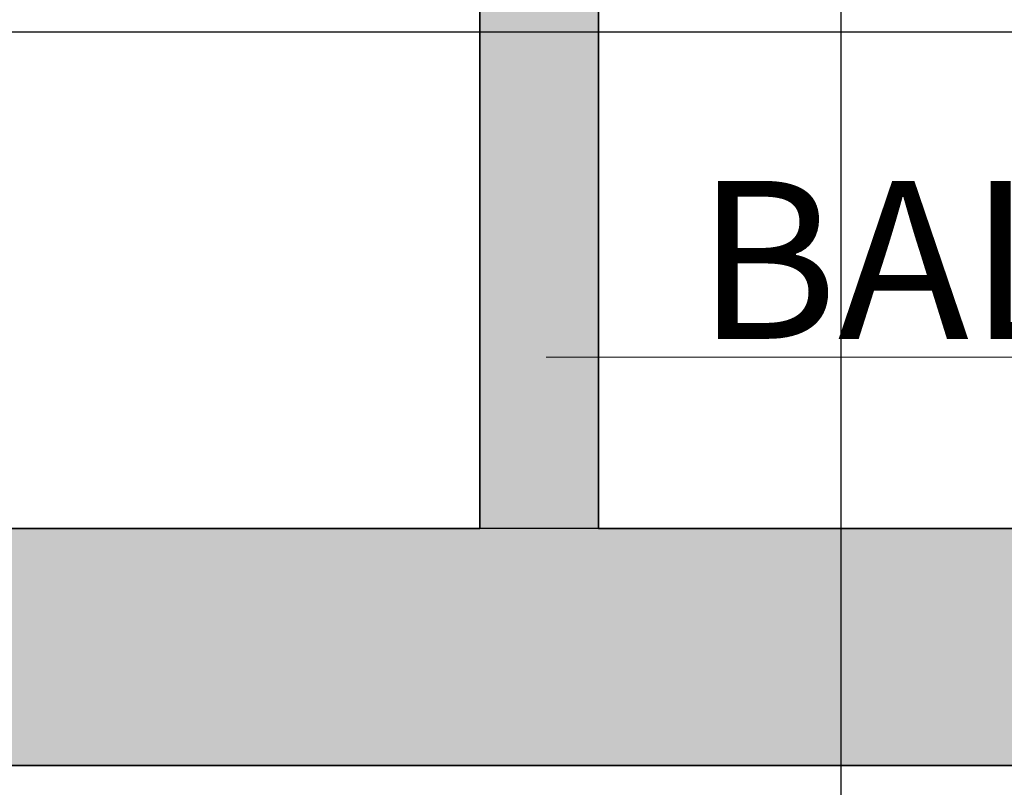
# Model space of a CAD drawing. Units: inches. Extents: x 2696 to 3240, y 1564 to 2310.
# Tile 3 of 76: x 2875 to 2912, y 1604 to 1634. Entities that reach past the tile are written whole.
import ezdxf

# ---------------------------------------------------------------- set-up
doc = ezdxf.new("R2010")
doc.units = ezdxf.units.IN
for name, color, linetype, lineweight in [('A-ANNO-DIMS', 3, 'Continuous', 18), ('A-WALL', 7, 'Continuous', 35), ('A-WALL-PATT', 9, 'Continuous', 13)]:
    doc.layers.add(name, color=color, linetype=linetype, lineweight=lineweight)
doc.styles.add('TIMES NEW', font='times.ttf')
doc.dimstyles.new('Siddhuu', dxfattribs={"dimtxt": 6, "dimasz": 2.5, "dimexe": 1.25, "dimexo": 0.625, "dimtad": 1, "dimdec": 1, "dimlunit": 4, "dimtxsty": 'TIMES NEW', "dimcen": 2.5, "dimclrd": 256, "dimclre": 1, "dimclrt": 7, "dimadec": 0, "dimazin": 0, "dimtfac": 1, "dimtdec": 1, "dimtmove": 0, "dimatfit": 3, "dimfxl": 1, "dimtolj": 1, "dimlwd": -1, "dimarcsym": 0})

# ---------------------------------------------------------------- blocks, each defined once
blk = doc.blocks.new('*D36')
at = {"layer": 'A-ANNO-DIMS', "color": 1, "lineweight": -2, "transparency": 16777216}
for p, q in [((3008.237, 1629.386), (3008.237, 1619.461)), ((3070.237, 1629.386), (3070.237, 1619.461))]:
    blk.add_line(p, q, dxfattribs=at)
at = {"layer": 'A-ANNO-DIMS', "transparency": 16777216}
for p, q in [((3008.237, 1620.711), (2894.718, 1620.711)), ((3067.737, 1620.711), (3010.737, 1620.711))]:
    blk.add_line(p, q, dxfattribs=at)
for points in [[(3010.737, 1621.128), (3010.737, 1620.294), (3008.237, 1620.711)], [(3067.737, 1621.128), (3067.737, 1620.294), (3070.237, 1620.711)]]:
    blk.add_solid(points, dxfattribs=at)
at = {"layer": 'Defpoints', "color": 0, "transparency": 16777216}
for p in [(3008.237, 1630.011), (3070.237, 1630.011), (3008.237, 1620.711)]:
    blk.add_point(p, dxfattribs=at)
at = {"layer": 'A-ANNO-DIMS', "color": 7, "transparency": 16777216, "insert": (2950.228, 1624.403), "char_height": 6, "attachment_point": 5, "style": 'TIMES NEW'}
blk.add_mtext('\\A1;BALCONY DOOR 5\'-2" TYP.', dxfattribs=at)
blk = doc.blocks.new('*D57')
at = {"layer": 'A-ANNO-DIMS', "color": 1, "lineweight": -2, "transparency": 16777216}
for p, q in [((2754.611, 2018.576), (2754.611, 1568.951)), ((2956.709, 2018.576), (2956.709, 1568.951))]:
    blk.add_line(p, q, dxfattribs=at)
at = {"layer": 'A-ANNO-DIMS', "transparency": 16777216}
blk.add_line((2757.111, 1570.201), (2954.209, 1570.201), dxfattribs=at)
for points in [[(2757.111, 1570.618), (2757.111, 1569.784), (2754.611, 1570.201)], [(2954.209, 1570.618), (2954.209, 1569.784), (2956.709, 1570.201)]]:
    blk.add_solid(points, dxfattribs=at)
at = {"layer": 'Defpoints', "color": 0, "transparency": 16777216}
for p in [(2754.611, 2019.201), (2956.709, 2019.201), (2956.709, 1570.201)]:
    blk.add_point(p, dxfattribs=at)
at = {"layer": 'A-ANNO-DIMS', "color": 7, "transparency": 16777216, "insert": (2855.66, 1573.878), "char_height": 6, "attachment_point": 5, "style": 'TIMES NEW'}
blk.add_mtext('\\A1;16\'-10"', dxfattribs=at)
blk = doc.blocks.new('*D69')
at = {"layer": 'A-ANNO-DIMS', "color": 1, "lineweight": -2, "transparency": 16777216}
for p, q in [((2841.889, 2261.576), (2841.889, 1568.951)), ((2905.91, 2261.576), (2905.91, 1568.951))]:
    blk.add_line(p, q, dxfattribs=at)
at = {"layer": 'A-ANNO-DIMS', "transparency": 16777216}
blk.add_line((2844.389, 1570.201), (2903.41, 1570.201), dxfattribs=at)
for points in [[(2844.389, 1570.618), (2844.389, 1569.784), (2841.889, 1570.201)], [(2903.41, 1570.618), (2903.41, 1569.784), (2905.91, 1570.201)]]:
    blk.add_solid(points, dxfattribs=at)
at = {"layer": 'Defpoints', "color": 0, "transparency": 16777216}
for p in [(2841.889, 2262.201), (2905.91, 2262.201), (2905.91, 1570.201)]:
    blk.add_point(p, dxfattribs=at)
at = {"layer": 'A-ANNO-DIMS', "color": 7, "transparency": 16777216, "insert": (2873.9, 1573.878), "char_height": 6, "attachment_point": 5, "style": 'TIMES NEW'}
blk.add_mtext('\\A1;5\'-4"', dxfattribs=at)
blk = doc.blocks.new('*D81')
at = {"layer": 'A-ANNO-DIMS', "color": 1, "lineweight": -2, "transparency": 16777216}
for p, q in [((3189.986, 1633.048), (2709.361, 1633.048)), ((3189.986, 1614.201), (2709.361, 1614.201))]:
    blk.add_line(p, q, dxfattribs=at)
at = {"layer": 'A-ANNO-DIMS', "transparency": 16777216}
blk.add_line((2710.611, 1616.701), (2710.611, 1630.548), dxfattribs=at)
for points in [[(2710.195, 1630.548), (2711.028, 1630.548), (2710.611, 1633.048)], [(2710.195, 1616.701), (2711.028, 1616.701), (2710.611, 1614.201)]]:
    blk.add_solid(points, dxfattribs=at)
at = {"layer": 'Defpoints', "color": 0, "transparency": 16777216}
for p in [(2710.611, 1633.048), (3190.611, 1633.048), (3190.611, 1614.201)]:
    blk.add_point(p, dxfattribs=at)
at = {"layer": 'A-ANNO-DIMS', "color": 7, "transparency": 16777216, "insert": (2706.926, 1623.624), "char_height": 6, "attachment_point": 5, "rotation": 90, "style": 'TIMES NEW'}
blk.add_mtext('\\A1;1\'-7"', dxfattribs=at)

msp = doc.modelspace()

# ---------------------------------------------------------------- hatches: boundary and pattern name
at = {"layer": 'A-WALL-PATT', "transparency": 33554556}
h = msp.add_hatch(color=256, dxfattribs=at)
h.dxf.hatch_style = 1
h.paths.add_polyline_path([(2879.111, 2253.201), (2905.91, 2253.201), (2905.91, 2262.201), (2841.889, 2262.201), (2841.889, 2253.201), (2870.111, 2253.201), (2870.111, 2176.601), (2965.709, 2176.601), (2965.709, 2206.701), (2973.583, 2206.701), (2973.583, 2215.701), (2965.709, 2215.701), (2965.709, 2262.201), (2929.91, 2262.201), (2929.91, 2253.201), (2956.709, 2253.201), (2956.709, 2185.601), (2879.111, 2185.601)])
h.paths.add_polyline_path([(2782.834, 2262.201), (2745.611, 2262.201), (2745.611, 2228.729), (2754.611, 2228.729), (2754.611, 2253.201), (2782.834, 2253.201)])
h.paths.add_polyline_path([(2754.611, 2136.201), (2965.709, 2136.201), (2965.709, 2145.201), (2879.111, 2145.201), (2879.111, 2147.074), (2877.34, 2147.074), (2870.111, 2147.074), (2870.111, 2145.201), (2754.611, 2145.201), (2754.611, 2169.674), (2745.611, 2169.674), (2745.611, 2000.201), (2754.611, 2000.201), (2754.611, 2019.201), (2849.083, 2019.201), (2849.083, 2023.701), (2841.209, 2023.701), (2841.209, 2051.827), (2836.709, 2051.827), (2836.709, 2023.701), (2754.611, 2023.701), (2754.611, 2091.201), (2836.709, 2091.201), (2836.709, 2087.827), (2841.209, 2087.827), (2841.209, 2095.701), (2754.611, 2095.701)])
h.paths.add_polyline_path([(2965.709, 2136.201), (2956.709, 2136.201), (2956.709, 2023.701), (2885.083, 2023.701), (2885.083, 2019.201), (2956.709, 2019.201), (2956.709, 1950.575), (2965.709, 1950.575), (2965.709, 1980.201), (2973.583, 1980.201), (2973.583, 1989.201), (2965.709, 1989.201)])
h.paths.add_polyline_path([(2754.611, 1906.701), (2880.209, 1906.701), (2884.709, 1906.701), (2956.709, 1906.701), (2956.709, 1792.701), (2944.709, 1792.701), (2944.709, 1783.701), (2956.709, 1783.701), (2956.709, 1740.201), (2884.709, 1740.201), (2884.709, 1783.701), (2896.709, 1783.701), (2896.709, 1792.701), (2884.709, 1792.701), (2884.709, 1846.701), (2880.209, 1846.701), (2880.209, 1740.201), (2754.611, 1740.201), (2754.611, 1777.201), (2745.611, 1777.201), (2745.611, 1692.701), (2754.611, 1692.701), (2754.611, 1731.201), (2956.709, 1731.201), (2956.709, 1723.327), (2965.709, 1723.327), (2965.709, 1884.201), (2973.583, 1884.201), (2973.583, 1893.201), (2965.709, 1893.201), (2965.709, 1914.575), (2956.709, 1914.575), (2956.709, 1911.201), (2754.611, 1911.201), (2754.611, 1930.201), (2745.611, 1930.201), (2745.611, 1817.201), (2754.611, 1817.201), (2754.611, 1854.201), (2826.611, 1854.201), (2826.611, 1868.827), (2822.111, 1868.827), (2822.111, 1858.701), (2754.611, 1858.701)])
h.paths.add_polyline_path([(2965.709, 1656.201), (3008.237, 1656.201), (3008.237, 1665.201), (2965.709, 1665.201), (2965.709, 1693.327), (2956.709, 1693.327), (2956.709, 1686.201), (2934.583, 1686.201), (2934.583, 1681.701), (2956.709, 1681.701), (2956.709, 1614.201), (2896.709, 1614.201), (2896.709, 1681.701), (2904.583, 1681.701), (2904.583, 1686.201), (2892.209, 1686.201), (2892.209, 1614.201), (2858.41, 1614.201), (2858.41, 1605.201), (2965.709, 1605.201)])
h.paths.add_polyline_path([(2788.41, 1614.201), (2754.611, 1614.201), (2754.611, 1652.701), (2745.611, 1652.701), (2745.611, 1605.201), (2788.41, 1605.201)])
h.paths.add_polyline_path([(3199.611, 1633.048), (3190.611, 1633.048), (3190.611, 1614.201), (3082.611, 1614.201), (3082.611, 1665.201), (3070.237, 1665.201), (3070.237, 1656.201), (3078.111, 1656.201), (3078.111, 1605.201), (3199.611, 1605.201)])
h.paths.add_polyline_path([(3199.611, 1702.048), (3190.611, 1702.048), (3190.611, 1699.701), (3106.611, 1699.701), (3106.611, 1747.701), (3190.611, 1747.701), (3190.611, 1752.201), (3082.611, 1752.201), (3082.611, 1760.075), (3078.111, 1760.075), (3078.111, 1747.701), (3102.111, 1747.701), (3102.111, 1699.701), (3078.111, 1699.701), (3078.111, 1695.201), (3190.611, 1695.201), (3190.611, 1676.355), (3199.611, 1676.355)])
h.paths.add_polyline_path([(3199.611, 1783.201), (3190.611, 1783.201), (3190.611, 1745.355), (3199.611, 1745.355)])
h.paths.add_polyline_path([(3082.611, 1884.201), (3190.611, 1884.201), (3190.611, 1853.201), (3199.611, 1853.201), (3199.611, 1901.701), (3190.611, 1901.701), (3190.611, 1893.201), (3005.583, 1893.201), (3005.583, 1891.281), (3005.583, 1884.201), (3078.111, 1884.201), (3078.111, 1792.075), (3082.611, 1792.075)])
h.paths.add_polyline_path([(3199.611, 1994.701), (3190.611, 1994.701), (3190.611, 1989.201), (3073.709, 1989.201), (3073.709, 2034.201), (3069.209, 2034.201), (3069.209, 1989.201), (3005.583, 1989.201), (3005.583, 1980.201), (3190.611, 1980.201), (3190.611, 1971.701), (3199.611, 1971.701)])
h.paths.add_polyline_path([(3199.611, 2155.201), (3190.611, 2155.201), (3190.611, 2064.701), (3199.611, 2064.701)])
h.paths.add_polyline_path([(3190.611, 2074.701), (3106.611, 2074.701), (3106.611, 2122.701), (3190.611, 2122.701), (3190.611, 2127.201), (3082.709, 2127.201), (3082.709, 2135.075), (3073.709, 2135.075), (3073.709, 2122.701), (3102.111, 2122.701), (3102.111, 2074.701), (3069.209, 2074.701), (3069.209, 2070.201), (3190.611, 2070.201)])
h.paths.add_polyline_path([(3082.709, 2253.201), (3190.611, 2253.201), (3190.611, 2225.201), (3199.611, 2225.201), (3199.611, 2262.201), (3073.709, 2262.201), (3073.709, 2215.701), (3035.583, 2215.701), (3035.583, 2206.701), (3073.709, 2206.701), (3073.709, 2171.075), (3082.709, 2171.075)])

# ---------------------------------------------------------------- linework, layer by layer
at = {"layer": 'A-WALL'}
for p, q in [((2892.209, 1686.201), (2892.209, 1614.201)), ((2896.709, 1681.701), (2896.709, 1614.201)), ((2858.41, 1614.201), (2892.209, 1614.201)), ((2896.709, 1614.201), (2956.709, 1614.201)), ((2858.41, 1605.201), (2965.709, 1605.201))]:
    msp.add_line(p, q, dxfattribs=at)

# ---------------------------------------------------------------- dimensions: what is measured, and where the dimension line sits
at = {"layer": 'A-ANNO-DIMS'}
for base, p1, p2, picture, middle in [((2905.91, 1570.201), (2841.889, 2262.201), (2905.91, 2262.201), '*D69', (2873.9, 1573.878)), ((2956.709, 1570.201), (2754.611, 2019.201), (2956.709, 2019.201), '*D57', (2855.66, 1573.878))]:
    dim = msp.add_linear_dim(base=base, p1=p1, p2=p2, dimstyle='Siddhuu', override={"dimdec": 1, "dimlfac": 1, "dimrnd": 0, "dimzin": 1, "dimdsep": 46, "dimlunit": 4, "dimfrac": 2}, dxfattribs=at)
    dim.commit()
    dim.dimension.update_dxf_attribs({"geometry": picture, "text_midpoint": middle})
dim = msp.add_linear_dim(base=(3008.237, 1620.711), p1=(3070.237, 1630.011), p2=(3008.237, 1630.011), angle=180, text='BALCONY DOOR <> TYP.', dimstyle='Siddhuu', override={"dimdec": 1, "dimlfac": 1, "dimrnd": 0, "dimzin": 1, "dimdsep": 46, "dimlunit": 4, "dimfrac": 2}, dxfattribs=at)
dim.commit()
dim.dimension.update_dxf_attribs({"geometry": '*D36', "text_midpoint": (2950.228, 1624.403)})
dim = msp.add_linear_dim(base=(2710.611, 1633.048), p1=(3190.611, 1614.201), p2=(3190.611, 1633.048), angle=90, dimstyle='Siddhuu', override={"dimdec": 1, "dimlfac": 1, "dimrnd": 0, "dimzin": 1, "dimdsep": 46, "dimlunit": 4, "dimfrac": 2}, dxfattribs=at)
dim.commit()
dim.dimension.update_dxf_attribs({"geometry": '*D81', "text_midpoint": (2706.926, 1623.624)})

doc.saveas('drawing.dxf')
